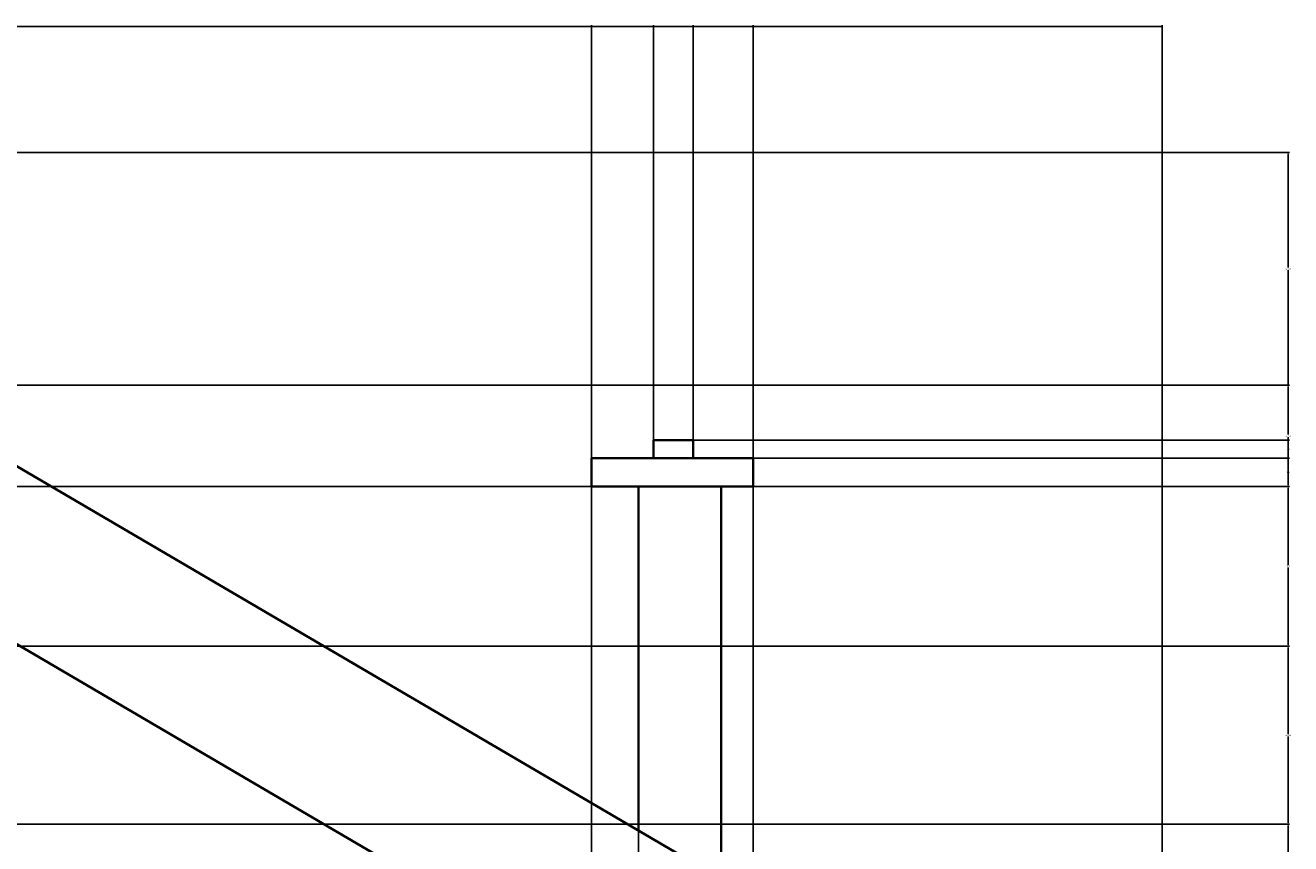
# Model space of a CAD drawing. Units: inches. Extents: x 27 to 409, y -26 to 294.
# Tile 7 of 7: x 230 to 409, y 178 to 294. Entities that reach past the tile are written whole.
import ezdxf

# ---------------------------------------------------------------- set-up
doc = ezdxf.new("R2010")
doc.units = ezdxf.units.IN
doc.header["$MEASUREMENT"] = 0
doc.layers.add('A-ANNO-DIMS', color=2, linetype='Continuous', lineweight=18)
doc.layers.add('A-ROOF', color=1, linetype='Continuous', lineweight=35)
doc.styles.get("Standard").update_dxf_attribs({"font": 'arial.ttf'})
doc.dimstyles.get("Standard").update_dxf_attribs({"dimtxt": 0.18, "dimasz": 0.18, "dimexe": 0.18, "dimexo": 0.0625, "dimgap": 0.09, "dimtad": 0, "dimtih": 1, "dimtoh": 1, "dimdec": 4, "dimzin": 0, "dimdsep": 46, "dimtxsty": 'Standard', "dimcen": 0.09, "dimadec": 0, "dimazin": 0, "dimtfac": 1, "dimtdec": 4, "dimtofl": 0, "dimtmove": 0, "dimatfit": 3, "dimfxl": 1, "dimtolj": 1, "dimtzin": 0, "dimarcsym": 0})

# ---------------------------------------------------------------- blocks, each defined once
blk = doc.blocks.new('*D7')
at = {"layer": 'A-ANNO-DIMS', "color": 0, "lineweight": -2, "transparency": 16777216}
for p, q in [((45.58, 108.44), (45.58, 293.63)), ((45.76, 293.45), (217.77, 293.45)), ((390.53, 293.45), (218.52, 293.45)), ((390.71, 136.32), (390.71, 293.63))]:
    blk.add_line(p, q, dxfattribs=at)
at = {"layer": 'A-ANNO-DIMS', "color": 0, "transparency": 16777216}
for points in [[(45.76, 293.48), (45.76, 293.42), (45.58, 293.45)], [(390.53, 293.48), (390.53, 293.42), (390.71, 293.45)]]:
    blk.add_solid(points, dxfattribs=at)
at = {"layer": 'Defpoints', "color": 0, "transparency": 16777216}
for p in [(390.71, 293.45), (390.71, 136.26), (45.58, 108.38)]:
    blk.add_point(p, dxfattribs=at)
at = {"layer": 'A-ANNO-DIMS', "color": 0, "transparency": 16777216, "insert": (218.14, 293.45), "char_height": 0.18, "attachment_point": 5}
blk.add_mtext('\\A1;345.1', dxfattribs=at)
blk = doc.blocks.new('*D44')
at = {"layer": 'A-ANNO-DIMS', "color": 0, "lineweight": -2, "transparency": 16777216}
for p, q in [((166.14, 180.59), (408.69, 180.59)), ((408.51, 180.41), (408.51, 158.6)), ((408.51, 136.44), (408.51, 158.24)), ((390.77, 136.26), (408.69, 136.26))]:
    blk.add_line(p, q, dxfattribs=at)
at = {"layer": 'A-ANNO-DIMS', "color": 0, "transparency": 16777216}
for points in [[(408.48, 180.41), (408.54, 180.41), (408.51, 180.59)], [(408.48, 136.44), (408.54, 136.44), (408.51, 136.26)]]:
    blk.add_solid(points, dxfattribs=at)
at = {"layer": 'Defpoints', "color": 0, "transparency": 16777216}
for p in [(166.08, 180.59), (408.51, 180.59), (390.71, 136.26)]:
    blk.add_point(p, dxfattribs=at)
at = {"layer": 'A-ANNO-DIMS', "color": 0, "transparency": 16777216, "insert": (408.51, 158.42), "char_height": 0.18, "attachment_point": 5}
blk.add_mtext('\\A1;44.33', dxfattribs=at)
blk = doc.blocks.new('*D45')
at = {"layer": 'A-ANNO-DIMS', "color": 0, "lineweight": -2, "transparency": 16777216}
for p, q in [((166.14, 205.78), (408.69, 205.78)), ((408.51, 205.6), (408.51, 193.36)), ((408.51, 180.77), (408.51, 193)), ((166.14, 180.59), (408.69, 180.59))]:
    blk.add_line(p, q, dxfattribs=at)
at = {"layer": 'A-ANNO-DIMS', "color": 0, "transparency": 16777216}
for points in [[(408.48, 205.6), (408.54, 205.6), (408.51, 205.78)], [(408.48, 180.77), (408.54, 180.77), (408.51, 180.59)]]:
    blk.add_solid(points, dxfattribs=at)
at = {"layer": 'Defpoints', "color": 0, "transparency": 16777216}
for p in [(166.08, 205.78), (408.51, 205.78), (166.08, 180.59)]:
    blk.add_point(p, dxfattribs=at)
at = {"layer": 'A-ANNO-DIMS', "color": 0, "transparency": 16777216, "insert": (408.51, 193.18), "char_height": 0.18, "attachment_point": 5}
blk.add_mtext('\\A1;25.194', dxfattribs=at)
blk = doc.blocks.new('*D46')
at = {"layer": 'A-ANNO-DIMS', "color": 0, "lineweight": -2, "transparency": 16777216}
for p, q in [((190.14, 228.38), (408.69, 228.38)), ((408.51, 228.2), (408.51, 217.26)), ((408.51, 205.96), (408.51, 216.9)), ((166.14, 205.78), (408.69, 205.78))]:
    blk.add_line(p, q, dxfattribs=at)
at = {"layer": 'A-ANNO-DIMS', "color": 0, "transparency": 16777216}
for points in [[(408.48, 228.2), (408.54, 228.2), (408.51, 228.38)], [(408.48, 205.96), (408.54, 205.96), (408.51, 205.78)]]:
    blk.add_solid(points, dxfattribs=at)
at = {"layer": 'Defpoints', "color": 0, "transparency": 16777216}
for p in [(190.08, 228.38), (408.51, 228.38), (166.08, 205.78)]:
    blk.add_point(p, dxfattribs=at)
at = {"layer": 'A-ANNO-DIMS', "color": 0, "transparency": 16777216, "insert": (408.51, 217.08), "char_height": 0.18, "attachment_point": 5}
blk.add_mtext('\\A1;22.6', dxfattribs=at)
blk = doc.blocks.new('*D47')
at = {"layer": 'A-ANNO-DIMS', "color": 0, "lineweight": -2, "transparency": 16777216}
for p, q in [((166.14, 242.7), (408.69, 242.7)), ((408.51, 242.52), (408.51, 235.72)), ((408.51, 228.56), (408.51, 235.36)), ((190.14, 228.38), (408.69, 228.38))]:
    blk.add_line(p, q, dxfattribs=at)
at = {"layer": 'A-ANNO-DIMS', "color": 0, "transparency": 16777216}
for points in [[(408.48, 242.52), (408.54, 242.52), (408.51, 242.7)], [(408.48, 228.56), (408.54, 228.56), (408.51, 228.38)]]:
    blk.add_solid(points, dxfattribs=at)
at = {"layer": 'Defpoints', "color": 0, "transparency": 16777216}
for p in [(166.08, 242.7), (408.51, 242.7), (190.08, 228.38)]:
    blk.add_point(p, dxfattribs=at)
at = {"layer": 'A-ANNO-DIMS', "color": 0, "transparency": 16777216, "insert": (408.51, 235.54), "char_height": 0.18, "attachment_point": 5}
blk.add_mtext('\\A1;14.318', dxfattribs=at)
blk = doc.blocks.new('*D48')
at = {"layer": 'A-ANNO-DIMS', "color": 0, "lineweight": -2, "transparency": 16777216}
for p, q in [((152.9, 275.65), (408.69, 275.65)), ((408.51, 275.47), (408.51, 259.36)), ((408.51, 242.88), (408.51, 258.99)), ((166.14, 242.7), (408.69, 242.7))]:
    blk.add_line(p, q, dxfattribs=at)
at = {"layer": 'A-ANNO-DIMS', "color": 0, "transparency": 16777216}
for points in [[(408.48, 275.47), (408.54, 275.47), (408.51, 275.65)], [(408.48, 242.88), (408.54, 242.88), (408.51, 242.7)]]:
    blk.add_solid(points, dxfattribs=at)
at = {"layer": 'Defpoints', "color": 0, "transparency": 16777216}
for p in [(152.83, 275.65), (408.51, 275.65), (166.08, 242.7)]:
    blk.add_point(p, dxfattribs=at)
at = {"layer": 'A-ANNO-DIMS', "color": 0, "transparency": 16777216, "insert": (408.51, 259.17), "char_height": 0.18, "attachment_point": 5}
blk.add_mtext('\\A1;32.954', dxfattribs=at)
blk = doc.blocks.new('*D82')
at = {"layer": 'A-ANNO-DIMS', "color": 0, "lineweight": -2, "transparency": 16777216}
for p, q in [((309.93, 228.32), (309.93, -26.5)), ((316.59, 228.32), (316.59, -26.5)), ((310.11, -26.32), (312.86, -26.32)), ((316.41, -26.32), (313.65, -26.32))]:
    blk.add_line(p, q, dxfattribs=at)
at = {"layer": 'A-ANNO-DIMS', "color": 0, "transparency": 16777216}
for points in [[(310.11, -26.29), (310.11, -26.35), (309.93, -26.32)], [(316.41, -26.29), (316.41, -26.35), (316.59, -26.32)]]:
    blk.add_solid(points, dxfattribs=at)
at = {"layer": 'Defpoints', "color": 0, "transparency": 16777216}
for p in [(309.93, 228.38), (316.59, 228.38), (316.59, -26.32)]:
    blk.add_point(p, dxfattribs=at)
at = {"layer": 'A-ANNO-DIMS', "color": 0, "transparency": 16777216, "insert": (313.26, -26.32), "char_height": 0.18, "attachment_point": 5}
blk.add_mtext('\\A1;6.665', dxfattribs=at)
blk = doc.blocks.new('*D83')
at = {"layer": 'A-ANNO-DIMS', "color": 0, "lineweight": -2, "transparency": 16777216}
for p, q in [((316.59, 228.32), (316.59, -26.5)), ((328.29, 228.32), (328.29, -26.5)), ((316.77, -26.32), (321.99, -26.32)), ((328.11, -26.32), (322.9, -26.32))]:
    blk.add_line(p, q, dxfattribs=at)
at = {"layer": 'A-ANNO-DIMS', "color": 0, "transparency": 16777216}
for points in [[(316.77, -26.29), (316.77, -26.35), (316.59, -26.32)], [(328.11, -26.29), (328.11, -26.35), (328.29, -26.32)]]:
    blk.add_solid(points, dxfattribs=at)
at = {"layer": 'Defpoints', "color": 0, "transparency": 16777216}
for p in [(316.59, 228.38), (328.29, 228.38), (328.29, -26.32)]:
    blk.add_point(p, dxfattribs=at)
at = {"layer": 'A-ANNO-DIMS', "color": 0, "transparency": 16777216, "insert": (322.44, -26.32), "char_height": 0.18, "attachment_point": 5}
blk.add_mtext('\\A1;11.699', dxfattribs=at)
blk = doc.blocks.new('*D84')
at = {"layer": 'A-ANNO-DIMS', "color": 0, "lineweight": -2, "transparency": 16777216}
for p, q in [((328.29, 228.32), (328.29, -26.5)), ((332.8, 228.32), (332.8, -26.5)), ((328.47, -26.32), (330.17, -26.32)), ((332.62, -26.32), (330.93, -26.32))]:
    blk.add_line(p, q, dxfattribs=at)
at = {"layer": 'A-ANNO-DIMS', "color": 0, "transparency": 16777216}
for points in [[(328.47, -26.29), (328.47, -26.35), (328.29, -26.32)], [(332.62, -26.29), (332.62, -26.35), (332.8, -26.32)]]:
    blk.add_solid(points, dxfattribs=at)
at = {"layer": 'Defpoints', "color": 0, "transparency": 16777216}
for p in [(328.29, 228.38), (332.8, 228.38), (332.8, -26.32)]:
    blk.add_point(p, dxfattribs=at)
at = {"layer": 'A-ANNO-DIMS', "color": 0, "transparency": 16777216, "insert": (330.55, -26.32), "char_height": 0.18, "attachment_point": 5}
blk.add_mtext('\\A1;4.511', dxfattribs=at)
blk = doc.blocks.new('*D85')
at = {"layer": 'A-ANNO-DIMS', "color": 0, "lineweight": -2, "transparency": 16777216}
for p, q in [((309.93, 232.43), (309.93, 293.63)), ((310.11, 293.45), (314, 293.45)), ((318.54, 293.45), (314.65, 293.45)), ((318.72, 235.02), (318.72, 293.63))]:
    blk.add_line(p, q, dxfattribs=at)
at = {"layer": 'A-ANNO-DIMS', "color": 0, "transparency": 16777216}
for points in [[(310.11, 293.48), (310.11, 293.42), (309.93, 293.45)], [(318.54, 293.48), (318.54, 293.42), (318.72, 293.45)]]:
    blk.add_solid(points, dxfattribs=at)
at = {"layer": 'Defpoints', "color": 0, "transparency": 16777216}
for p in [(318.72, 293.45), (318.72, 234.95), (309.93, 232.37)]:
    blk.add_point(p, dxfattribs=at)
at = {"layer": 'A-ANNO-DIMS', "color": 0, "transparency": 16777216, "insert": (314.32, 293.45), "char_height": 0.18, "attachment_point": 5}
blk.add_mtext('\\A1;8.79', dxfattribs=at)
blk = doc.blocks.new('*D86')
at = {"layer": 'A-ANNO-DIMS', "color": 0, "lineweight": -2, "transparency": 16777216}
for p, q in [((318.72, 235.02), (318.72, 293.63)), ((318.9, 293.45), (321.14, 293.45)), ((324.16, 293.45), (321.92, 293.45)), ((324.34, 235.02), (324.34, 293.63))]:
    blk.add_line(p, q, dxfattribs=at)
at = {"layer": 'A-ANNO-DIMS', "color": 0, "transparency": 16777216}
for points in [[(318.9, 293.48), (318.9, 293.42), (318.72, 293.45)], [(324.16, 293.48), (324.16, 293.42), (324.34, 293.45)]]:
    blk.add_solid(points, dxfattribs=at)
at = {"layer": 'Defpoints', "color": 0, "transparency": 16777216}
for p in [(324.34, 293.45), (318.72, 234.95), (324.34, 234.95)]:
    blk.add_point(p, dxfattribs=at)
at = {"layer": 'A-ANNO-DIMS', "color": 0, "transparency": 16777216, "insert": (321.53, 293.45), "char_height": 0.18, "attachment_point": 5}
blk.add_mtext('\\A1;5.624', dxfattribs=at)
blk = doc.blocks.new('*D87')
at = {"layer": 'A-ANNO-DIMS', "color": 0, "lineweight": -2, "transparency": 16777216}
for p, q in [((324.34, 235.02), (324.34, 293.63)), ((324.52, 293.45), (328.25, 293.45)), ((332.62, 293.45), (328.89, 293.45)), ((332.8, 232.43), (332.8, 293.63))]:
    blk.add_line(p, q, dxfattribs=at)
at = {"layer": 'A-ANNO-DIMS', "color": 0, "transparency": 16777216}
for points in [[(324.52, 293.48), (324.52, 293.42), (324.34, 293.45)], [(332.62, 293.48), (332.62, 293.42), (332.8, 293.45)]]:
    blk.add_solid(points, dxfattribs=at)
at = {"layer": 'Defpoints', "color": 0, "transparency": 16777216}
for p in [(332.8, 293.45), (324.34, 234.95), (332.8, 232.37)]:
    blk.add_point(p, dxfattribs=at)
at = {"layer": 'A-ANNO-DIMS', "color": 0, "transparency": 16777216, "insert": (328.57, 293.45), "char_height": 0.18, "attachment_point": 5}
blk.add_mtext('\\A1;8.46', dxfattribs=at)
blk = doc.blocks.new('*D88')
at = {"layer": 'A-ANNO-DIMS', "color": 0, "lineweight": -2, "transparency": 16777216}
for p, q in [((332.86, 232.37), (408.69, 232.37)), ((408.51, 232.19), (408.51, 230.56)), ((408.51, 228.56), (408.51, 230.19)), ((332.86, 228.38), (408.69, 228.38))]:
    blk.add_line(p, q, dxfattribs=at)
at = {"layer": 'A-ANNO-DIMS', "color": 0, "transparency": 16777216}
for points in [[(408.48, 232.19), (408.54, 232.19), (408.51, 232.37)], [(408.48, 228.56), (408.54, 228.56), (408.51, 228.38)]]:
    blk.add_solid(points, dxfattribs=at)
at = {"layer": 'Defpoints', "color": 0, "transparency": 16777216}
for p in [(332.8, 232.37), (408.51, 232.37), (332.8, 228.38)]:
    blk.add_point(p, dxfattribs=at)
at = {"layer": 'A-ANNO-DIMS', "color": 0, "transparency": 16777216, "insert": (408.51, 230.37), "char_height": 0.18, "attachment_point": 5}
blk.add_mtext('\\A1;3.99', dxfattribs=at)
blk = doc.blocks.new('*D89')
at = {"layer": 'A-ANNO-DIMS', "color": 0, "lineweight": -2, "transparency": 16777216}
for p, q in [((324.4, 234.95), (408.69, 234.95)), ((408.51, 234.77), (408.51, 233.84)), ((408.51, 232.55), (408.51, 233.48)), ((332.86, 232.37), (408.69, 232.37))]:
    blk.add_line(p, q, dxfattribs=at)
at = {"layer": 'A-ANNO-DIMS', "color": 0, "transparency": 16777216}
for points in [[(408.48, 234.77), (408.54, 234.77), (408.51, 234.95)], [(408.48, 232.55), (408.54, 232.55), (408.51, 232.37)]]:
    blk.add_solid(points, dxfattribs=at)
at = {"layer": 'Defpoints', "color": 0, "transparency": 16777216}
for p in [(324.34, 234.95), (408.51, 234.95), (332.8, 232.37)]:
    blk.add_point(p, dxfattribs=at)
at = {"layer": 'A-ANNO-DIMS', "color": 0, "transparency": 16777216, "insert": (408.51, 233.66), "char_height": 0.18, "attachment_point": 5}
blk.add_mtext('\\A1;2.588', dxfattribs=at)

msp = doc.modelspace()

# ---------------------------------------------------------------- linework, layer by layer
at = {"layer": 'A-ROOF'}
msp.add_line((316.5916, 179.6883), (316.5916, 228.3803), dxfattribs=at)
for points in [[(166.0751, 242.6981), (379.7157, 117.5036), (390.7054, 136.2572), (152.833, 275.6517)], [(309.9262, 228.3803), (328.2901, 228.3803), (328.2901, 172.8329)]]:
    msp.add_lwpolyline(points, dxfattribs=at)
for points in [[(318.717, 232.3658), (324.3409, 232.3658), (324.3409, 234.9538), (318.717, 234.9538)], [(309.9262, 228.3803), (332.8007, 228.3803), (332.8007, 232.3658), (309.9262, 232.3658)]]:
    msp.add_lwpolyline(points, close=True, dxfattribs=at)

# ---------------------------------------------------------------- dimensions: what is measured, and where the dimension line sits
at = {"layer": 'A-ANNO-DIMS'}
for base, p1, p2, override, picture, middle in [((390.7054, 293.4517), (45.5772, 108.3803), (390.7054, 136.2572), {"dimdec": 1, "dimlfac": 1, "dimrnd": 0, "dimzin": 0, "dimdsep": 46, "dimlunit": 2}, '*D7', (218.1413, 293.4517)), ((318.717, 293.4517), (309.9262, 232.3658), (318.717, 234.9538), {"dimdec": 2, "dimlfac": 1, "dimrnd": 0, "dimzin": 0, "dimdsep": 46, "dimlunit": 2}, '*D85', (314.3216, 293.4517)), ((324.3409, 293.4517), (318.717, 234.9538), (324.3409, 234.9538), {"dimdec": 3, "dimlfac": 1, "dimrnd": 0, "dimzin": 0, "dimdsep": 46, "dimlunit": 2}, '*D86', (321.5289, 293.4517)), ((332.8007, 293.4517), (324.3409, 234.9538), (332.8007, 232.3658), {"dimdec": 2, "dimlfac": 1, "dimrnd": 0, "dimzin": 0, "dimdsep": 46, "dimlunit": 2}, '*D87', (328.5708, 293.4517)), ((316.5916, -26.3175), (309.9262, 228.3803), (316.5916, 228.3803), {"dimdec": 3, "dimlfac": 1, "dimrnd": 0, "dimzin": 0, "dimdsep": 46, "dimlunit": 2}, '*D82', (313.2589, -26.3175)), ((328.29013, -26.31755), (316.59157, 228.38031), (328.29013, 228.38031), {"dimdec": 3, "dimlfac": 1, "dimrnd": 0, "dimzin": 0, "dimdsep": 46, "dimlunit": 2}, '*D83', (322.44085, -26.31755)), ((332.8007, -26.3175), (328.2901, 228.3803), (332.8007, 228.3803), {"dimdec": 3, "dimlfac": 1, "dimrnd": 0, "dimzin": 0, "dimdsep": 46, "dimlunit": 2}, '*D84', (330.5454, -26.3175))]:
    dim = msp.add_linear_dim(base=base, p1=p1, p2=p2, dimstyle='Standard', override=override, dxfattribs=at)
    dim.commit()
    dim.dimension.update_dxf_attribs({"geometry": picture, "text_midpoint": middle})
for base, p1, p2, override, picture, middle in [((408.5054, 275.6517), (166.0751, 242.6981), (152.833, 275.6517), {"dimdec": 3, "dimlfac": 1, "dimrnd": 0, "dimzin": 0, "dimdsep": 46, "dimlunit": 2}, '*D48', (408.5054, 259.1749)), ((408.5054, 242.6981), (190.0751, 228.3803), (166.0751, 242.6981), {"dimdec": 3, "dimlfac": 1, "dimrnd": 0, "dimzin": 0, "dimdsep": 46, "dimlunit": 2}, '*D47', (408.5054, 235.5392)), ((408.5054, 234.9538), (332.8007, 232.3658), (324.3409, 234.9538), {"dimdec": 3, "dimlfac": 1, "dimrnd": 0, "dimzin": 0, "dimdsep": 46, "dimlunit": 2}, '*D89', (408.5054, 233.6598)), ((408.5054, 232.3658), (332.8007, 228.3803), (332.8007, 232.3658), {"dimdec": 2, "dimlfac": 1, "dimrnd": 0, "dimzin": 0, "dimdsep": 46, "dimlunit": 2}, '*D88', (408.5054, 230.3731)), ((408.5054, 228.3803), (166.0751, 205.7788), (190.0751, 228.3803), {"dimdec": 1, "dimlfac": 1, "dimrnd": 0, "dimzin": 0, "dimdsep": 46, "dimlunit": 2}, '*D46', (408.5054, 217.0795)), ((408.5054, 205.7788), (166.0751, 180.5852), (166.0751, 205.7788), {"dimdec": 3, "dimlfac": 1, "dimrnd": 0, "dimzin": 0, "dimdsep": 46, "dimlunit": 2}, '*D45', (408.5054, 193.182)), ((408.5054, 180.5852), (390.7054, 136.2572), (166.0751, 180.5852), {"dimdec": 2, "dimlfac": 1, "dimrnd": 0, "dimzin": 0, "dimdsep": 46, "dimlunit": 2}, '*D44', (408.5054, 158.4212))]:
    dim = msp.add_linear_dim(base=base, p1=p1, p2=p2, angle=90, dimstyle='Standard', override=override, dxfattribs=at)
    dim.commit()
    dim.dimension.update_dxf_attribs({"geometry": picture, "text_midpoint": middle})

doc.saveas('drawing.dxf')
